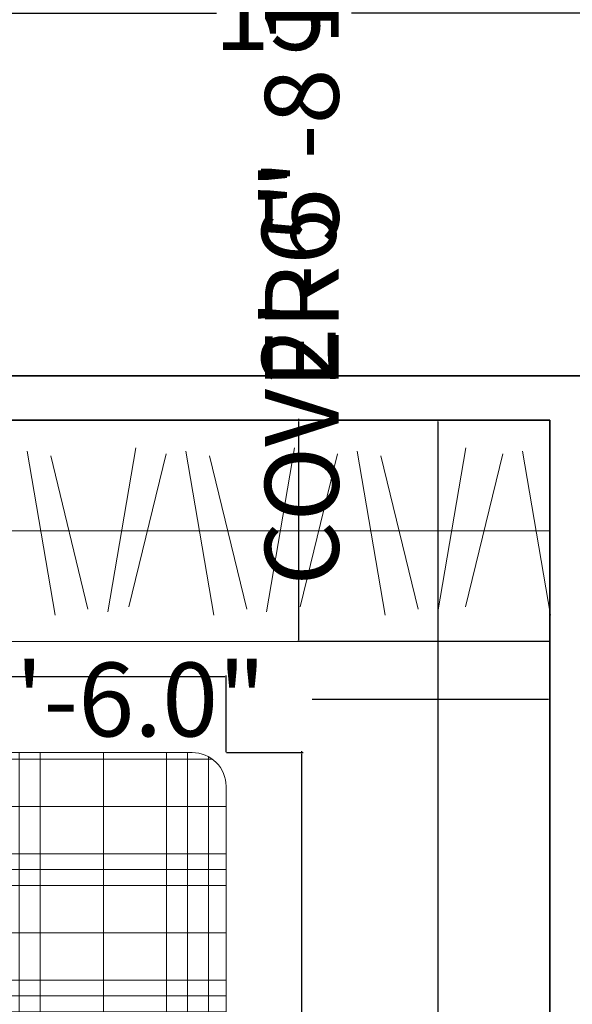
# Model space of a CAD drawing. Units: inches. Extents: x -269 to 4574, y -694 to 313.
# Tile 7 of 19: x 316 to 391, y -256 to -122. Entities that reach past the tile are written whole.
import ezdxf

# ---------------------------------------------------------------- set-up
doc = ezdxf.new("R2010")
doc.units = ezdxf.units.IN
doc.header["$MEASUREMENT"] = 0
for name, color, linetype, lineweight in [('A-FLOR-CASE', 2, 'Continuous', 18), ('A-FURN', 2, 'Continuous', 18), ('DIMENSION', 5, 'Continuous', 18), ('WALL', 1, 'Continuous', 35)]:
    doc.layers.add(name, color=color, linetype=linetype, lineweight=lineweight)
doc.dimstyles.get("Standard").update_dxf_attribs({"dimtxt": 10, "dimasz": 0.18, "dimexe": 0.18, "dimexo": 0.0625, "dimgap": 0.09, "dimtad": 0, "dimdec": 1, "dimzin": 0, "dimdsep": 46, "dimlunit": 3, "dimtxsty": 'Standard', "dimcen": 0.09, "dimclrt": 7, "dimadec": 0, "dimazin": 0, "dimtfac": 1, "dimtdec": 1, "dimtofl": 0, "dimtmove": 0, "dimatfit": 3, "dimfxl": 1, "dimtolj": 1, "dimtzin": 0, "dimarcsym": 0})

# ---------------------------------------------------------------- blocks, each defined once
blk = doc.blocks.new('*D20')
at = {"layer": 'Defpoints', "color": 0, "lineweight": 0, "transparency": 16777216}
for p in [(262.14, -122.44), (442.14, -121.56), (442.14, -122.44)]:
    blk.add_point(p, dxfattribs=at)
at = {"layer": 'DIMENSION', "color": 0, "lineweight": -2, "transparency": 16777216}
for p, q in [((262.14, -122.38), (262.14, -121.38)), ((442.14, -122.38), (442.14, -121.38)), ((262.32, -121.56), (343, -121.56)), ((441.96, -121.56), (361.27, -121.56))]:
    blk.add_line(p, q, dxfattribs=at)
at = {"layer": 'DIMENSION', "color": 0, "lineweight": 0, "transparency": 16777216}
for points in [[(262.32, -121.53), (262.32, -121.59), (262.14, -121.56)], [(441.96, -121.53), (441.96, -121.59), (442.14, -121.56)]]:
    blk.add_solid(points, dxfattribs=at)
at = {"layer": 'DIMENSION', "color": 0, "transparency": 16777216, "insert": (352.14, -121.56), "char_height": 10, "attachment_point": 5}
blk.add_mtext("\\A1;15'", dxfattribs=at)
blk = doc.blocks.new('*D21')
at = {"layer": 'Defpoints', "color": 0, "lineweight": 0, "transparency": 16777216}
for p in [(262.14, -206.73), (388.14, -206.73), (262.14, -214.6)]:
    blk.add_point(p, dxfattribs=at)
at = {"layer": 'DIMENSION', "color": 0, "lineweight": -2, "transparency": 16777216}
for p, q in [((262.14, -206.79), (262.14, -214.78)), ((388.14, -206.79), (388.14, -214.78)), ((262.32, -214.6), (294.33, -214.6)), ((387.96, -214.6), (355.94, -214.6))]:
    blk.add_line(p, q, dxfattribs=at)
at = {"layer": 'DIMENSION', "color": 0, "lineweight": 0, "transparency": 16777216}
for points in [[(262.32, -214.57), (262.32, -214.63), (262.14, -214.6)], [(387.96, -214.57), (387.96, -214.63), (388.14, -214.6)]]:
    blk.add_solid(points, dxfattribs=at)
at = {"layer": 'DIMENSION', "color": 0, "transparency": 16777216, "insert": (325.14, -214.6), "char_height": 10, "attachment_point": 5}
blk.add_mtext('\\A1;10\'-6.0"', dxfattribs=at)
blk = doc.blocks.new('*D22')
at = {"layer": 'Defpoints', "color": 0, "lineweight": 0, "transparency": 16777216}
for p in [(372.99, -176.73), (388.14, -176.73), (388.14, -356.73)]:
    blk.add_point(p, dxfattribs=at)
at = {"layer": 'DIMENSION', "color": 0, "lineweight": -2, "transparency": 16777216}
for p, q in [((388.07, -176.73), (372.81, -176.73)), ((372.99, -176.91), (372.99, -257.59)), ((372.99, -356.55), (372.99, -275.87)), ((388.07, -356.73), (372.81, -356.73))]:
    blk.add_line(p, q, dxfattribs=at)
at = {"layer": 'DIMENSION', "color": 0, "lineweight": 0, "transparency": 16777216}
for points in [[(372.96, -176.91), (373.02, -176.91), (372.99, -176.73)], [(372.96, -356.55), (373.02, -356.55), (372.99, -356.73)]]:
    blk.add_solid(points, dxfattribs=at)
at = {"layer": 'DIMENSION', "color": 0, "transparency": 16777216, "insert": (372.99, -266.73), "char_height": 10, "attachment_point": 5, "rotation": 90}
blk.add_mtext("\\A1;15'", dxfattribs=at)
blk = doc.blocks.new('*X10')
at = {"color": 0}
for p, q in [((276.598, 451.25), (280.51, 451.25)), ((275.455, 450.625), (280.51, 450.625)), ((274.411, 450), (280.51, 450)), ((265.51, 448.125), (267.634, 448.125)), ((271.723, 448.125), (280.51, 448.125)), ((265.51, 446.25), (268.465, 446.25)), ((269.519, 446.25), (280.51, 446.25)), ((265.51, 445.625), (268.531, 445.625)), ((268.866, 445.625), (280.51, 445.625)), ((265.51, 445), (280.51, 445)), ((265.51, 443.125), (280.51, 443.125)), ((265.51, 441.25), (280.51, 441.25)), ((265.51, 440.625), (280.51, 440.625)), ((265.634, 440), (280.386, 440))]:
    blk.add_line(p, q, dxfattribs=at)
blk = doc.blocks.new('*X11')
at = {"color": 0}
for p, q in [((280.312, 439.886), (280.312, 452.896)), ((278.906, 439.482), (278.906, 452.338)), ((277.5, 439.482), (277.5, 451.702)), ((276.562, 439.482), (276.562, 451.231)), ((277.031, 439.482), (277.031, 451.471)), ((275.156, 439.482), (275.156, 450.451)), ((265.781, 439.797), (265.781, 449.511)), ((273.75, 439.482), (273.75, 449.576)), ((266.25, 439.517), (266.25, 449.296)), ((273.281, 439.482), (273.281, 449.261)), ((272.812, 439.482), (272.812, 448.934)), ((267.656, 439.482), (267.656, 448.095)), ((271.406, 439.482), (271.406, 447.876)), ((270, 439.482), (270, 446.689)), ((269.531, 439.482), (269.531, 446.262)), ((269.062, 439.482), (269.062, 445.817))]:
    blk.add_line(p, q, dxfattribs=at)
blk = doc.blocks.new('BED-DOUBLE-COVER')
for centre, radius, start, end in [((63.32, -75.96), 137.6, 87.8642, 117.4001), ((118.65, -76.93), 147.29, 109.926, 135.3977), ((36.86, 17.25), 36.85, 94.4436, 133.2788), ((41.52, 23.74), 27.87, 97.2157, 147.6656), ((-5.92, 27.4), 19.71, 357.3792, 72.5379)]:
    blk.add_arc(centre, radius, start, end)
at = {"xscale": 4.5633847399786, "yscale": 4.5633847399786, "zscale": 4.5633847399786}
for name in ['*X11', '*X10']:
    blk.add_blockref(name, (-1211.62, -2005.53), dxfattribs=at)
blk = doc.blocks.new('*D49')
at = {"layer": 'Defpoints', "color": 0, "lineweight": 0, "transparency": 16777216}
for p in [(344.28, -221.79), (354.55, -221.79), (344.28, -290.24)]:
    blk.add_point(p, dxfattribs=at)
at = {"layer": 'DIMENSION', "color": 0, "lineweight": -2, "transparency": 16777216}
for p, q in [((344.34, -221.79), (354.73, -221.79)), ((354.55, -221.79), (354.55, -221.61)), ((354.55, -290.06), (354.55, -221.97)), ((344.34, -290.24), (354.73, -290.24))]:
    blk.add_line(p, q, dxfattribs=at)
at = {"layer": 'DIMENSION', "color": 0, "lineweight": 0, "transparency": 16777216}
for points in [[(354.52, -221.97), (354.58, -221.97), (354.55, -221.79)], [(354.52, -290.06), (354.58, -290.06), (354.55, -290.24)]]:
    blk.add_solid(points, dxfattribs=at)
at = {"layer": 'DIMENSION', "color": 7, "transparency": 16777216, "insert": (354.55, -133.67), "char_height": 10, "attachment_point": 5, "rotation": 90}
blk.add_mtext('\\A1;COVER 5\'-8 1/2" TYP.', dxfattribs=at)
blk = doc.blocks.new('*D50')
at = {"layer": 'Defpoints', "color": 0, "lineweight": 0, "transparency": 16777216}
for p in [(281.85, -211.53), (281.85, -221.79), (344.28, -221.79)]:
    blk.add_point(p, dxfattribs=at)
at = {"layer": 'DIMENSION', "color": 0, "lineweight": -2, "transparency": 16777216}
for p, q in [((281.85, -211.53), (281.67, -211.53)), ((281.85, -221.73), (281.85, -211.35)), ((344.1, -211.53), (282.03, -211.53)), ((344.28, -221.73), (344.28, -211.35))]:
    blk.add_line(p, q, dxfattribs=at)
at = {"layer": 'DIMENSION', "color": 0, "lineweight": 0, "transparency": 16777216}
for points in [[(282.03, -211.5), (282.03, -211.56), (281.85, -211.53)], [(344.1, -211.5), (344.1, -211.56), (344.28, -211.53)]]:
    blk.add_solid(points, dxfattribs=at)
at = {"layer": 'DIMENSION', "color": 7, "transparency": 16777216, "insert": (222.77, -211.53), "char_height": 10, "attachment_point": 5}
blk.add_mtext('\\A1;5\'-2 1/2" TYP.', dxfattribs=at)
blk = doc.blocks.new('*D80')
at = {"layer": 'Defpoints', "color": 0, "lineweight": 0, "transparency": 16777216}
for p in [(354.14, -176.73), (388.14, -176.73), (388.14, -206.73)]:
    blk.add_point(p, dxfattribs=at)
at = {"layer": 'DIMENSION', "color": 0, "lineweight": -2, "transparency": 16777216}
for p, q in [((388.07, -176.73), (353.96, -176.73)), ((354.14, -176.73), (354.14, -176.55)), ((354.14, -206.55), (354.14, -176.91)), ((388.07, -206.73), (353.96, -206.73))]:
    blk.add_line(p, q, dxfattribs=at)
at = {"layer": 'DIMENSION', "color": 0, "lineweight": 0, "transparency": 16777216}
for points in [[(354.11, -176.91), (354.17, -176.91), (354.14, -176.73)], [(354.11, -206.55), (354.17, -206.55), (354.14, -206.73)]]:
    blk.add_solid(points, dxfattribs=at)
at = {"layer": 'DIMENSION', "color": 7, "transparency": 16777216, "insert": (354.14, -156.7), "char_height": 10, "attachment_point": 5, "rotation": 90}
blk.add_mtext('\\A1;2\'-6"', dxfattribs=at)

msp = doc.modelspace()

# ---------------------------------------------------------------- linework, layer by layer
at = {"layer": 'A-FLOR-CASE'}
for p, q in [((388.14, -176.73), (388.14, -206.73)), ((321.13, -203.15), (317.34, -180.92)), ((332.06, -180.48), (328.27, -202.71)), ((331.11, -202.06), (336.15, -181.28)), ((342.63, -203.15), (338.84, -180.92)), ((353.56, -180.48), (349.77, -202.71)), ((354.33, -202.06), (359.37, -181.28)), ((365.84, -203.15), (362.05, -180.92)), ((376.78, -180.48), (372.99, -202.71)), ((376.74, -202.06), (381.78, -181.28)), ((388.25, -203.15), (384.46, -180.92)), ((320.54, -181.57), (325.58, -202.35)), ((342.04, -181.57), (347.09, -202.35)), ((365.26, -181.57), (370.3, -202.35)), ((388.14, -191.73), (262.14, -191.73)), ((262.14, -206.73), (388.14, -206.73))]:
    msp.add_line(p, q, dxfattribs=at)
at = {"layer": 'A-FURN'}
msp.add_lwpolyline([(344.28, -226.36), (344.28, -285.68, -0.414214), (339.71, -290.24), (266.7, -290.24, -0.414214), (262.14, -285.68), (262.14, -226.36, -0.414214), (266.7, -221.79), (339.71, -221.79, -0.414214)], format="xyb", close=True, dxfattribs=at)
at = {"layer": 'WALL'}
for p, q in [((262.14, -170.73), (394.14, -170.73)), ((262.14, -176.73), (388.14, -176.73)), ((388.14, -176.73), (388.14, -279.73))]:
    msp.add_line(p, q, dxfattribs=at)

# ---------------------------------------------------------------- block references
at = {"layer": 'A-FURN', "rotation": 90.00000000000024}
msp.add_blockref('BED-DOUBLE-COVER', (344.28, -290.24), dxfattribs=at)

# ---------------------------------------------------------------- dimensions: what is measured, and where the dimension line sits
at = {"layer": 'DIMENSION'}
for base, p1, p2, angle, text, picture, middle in [((354.5455, -221.7935), (344.2779, -290.2443), (344.2779, -221.7935), 90, 'COVER <> TYP.', '*D49', (354.5455, -133.6663)), ((281.85, -211.53), (344.28, -221.79), (281.85, -221.79), 180, '<> TYP.', '*D50', (222.77, -211.53))]:
    dim = msp.add_linear_dim(base=base, p1=p1, p2=p2, angle=angle, text=text, dimstyle='Standard', override={"dimdec": 1, "dimlfac": 1, "dimrnd": 0, "dimzin": 1, "dimdsep": 46, "dimlunit": 4, "dimfrac": 2}, dxfattribs=at)
    dim.commit()
    dim.dimension.update_dxf_attribs({"geometry": picture, "text_midpoint": middle})
for base, p1, p2, picture, middle in [((442.14, -121.56), (262.14, -122.44), (442.14, -122.44), '*D20', (352.14, -121.56)), ((262.14, -214.6), (388.14, -206.73), (262.14, -206.73), '*D21', (325.14, -214.6))]:
    dim = msp.add_linear_dim(base=base, p1=p1, p2=p2, dimstyle='Standard', override={"dimclrd": 0, "dimclre": 0, "dimclrt": 0}, dxfattribs=at)
    dim.commit()
    dim.dimension.update_dxf_attribs({"geometry": picture, "text_midpoint": middle})
for base, p1, override, picture, middle in [((354.14, -176.73), (388.14, -206.73), {"dimdec": 1, "dimlfac": 1, "dimrnd": 0, "dimzin": 1, "dimdsep": 46, "dimlunit": 4, "dimfrac": 2}, '*D80', (354.14, -156.7)), ((372.99, -176.73), (388.14, -356.73), {"dimclrd": 0, "dimclre": 0, "dimclrt": 0}, '*D22', (372.99, -266.73))]:
    dim = msp.add_linear_dim(base=base, p1=p1, p2=(388.14, -176.73), angle=90, dimstyle='Standard', override=override, dxfattribs=at)
    dim.commit()
    dim.dimension.update_dxf_attribs({"geometry": picture, "text_midpoint": middle})

doc.saveas('drawing.dxf')
